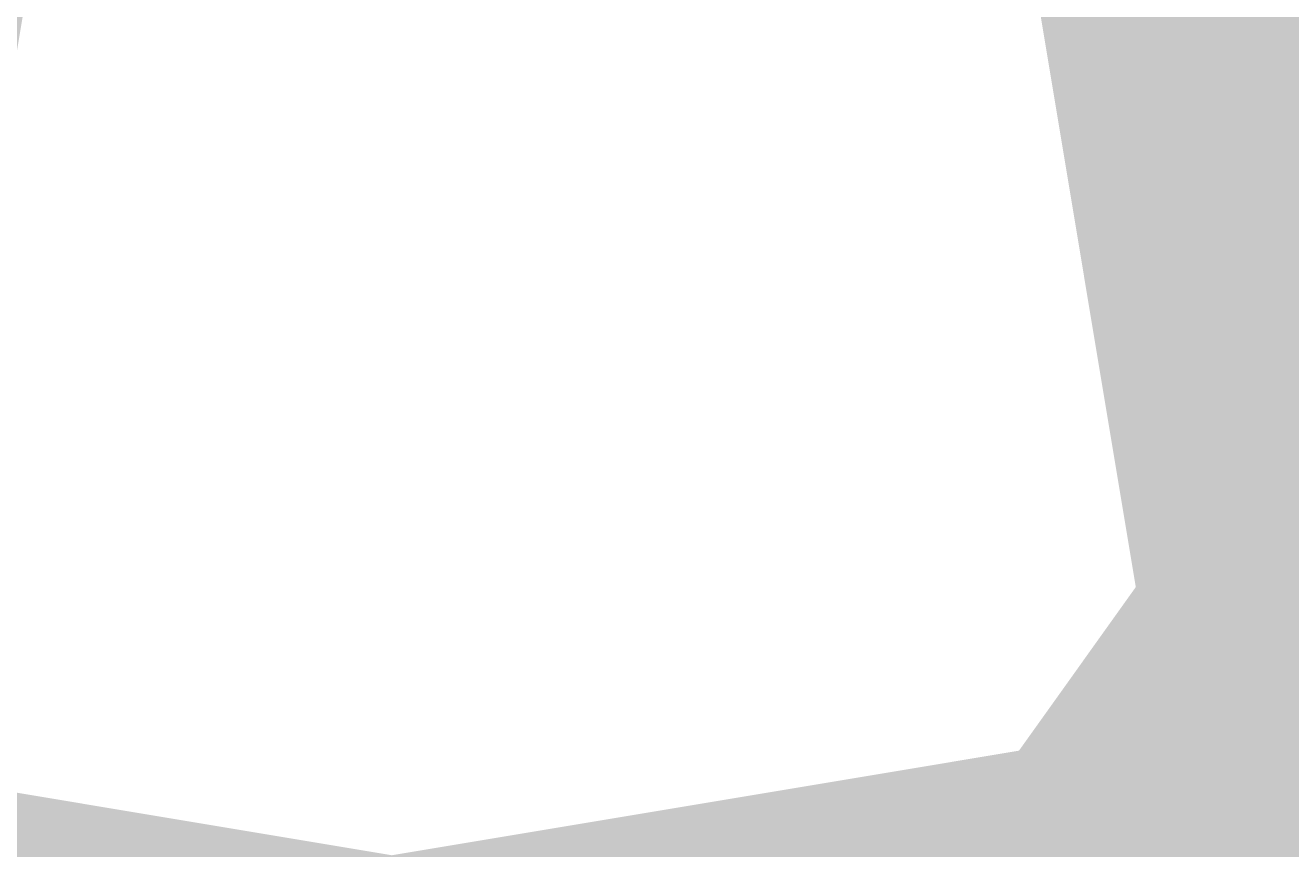
# Model space of a CAD drawing. Units: millimetres. Extents: x -22994 to 29398, y -19990 to 20176.
# Tile 122 of 135: x 99 to 296, y 213 to 341. Entities that reach past the tile are written whole.
import ezdxf

# ---------------------------------------------------------------- set-up
doc = ezdxf.new("R2010")
doc.units = ezdxf.units.MM
doc.header["$MEASUREMENT"] = 0
doc.layers.add('M-DIMS', color=2, linetype='Continuous', lineweight=18)
doc.styles.get("Standard").update_dxf_attribs({"font": 'arial.ttf'})
doc.dimstyles.get("Standard").update_dxf_attribs({"dimtxt": 0.18, "dimasz": 10000, "dimexe": 0.18, "dimexo": 0.0625, "dimgap": 0.09, "dimtad": 0, "dimtih": 1, "dimtoh": 1, "dimdec": 0, "dimzin": 0, "dimdsep": 46, "dimtxsty": 'Standard', "dimcen": 0.09, "dimadec": 0, "dimazin": 0, "dimtfac": 1, "dimtdec": 0, "dimtofl": 0, "dimtmove": 0, "dimatfit": 3, "dimfxl": 1, "dimtolj": 1, "dimtzin": 0, "dimlwd": 30, "dimarcsym": 0})

# ---------------------------------------------------------------- blocks, each defined once
blk = doc.blocks.new('*D2')
at = {"layer": 'Defpoints', "color": 0, "transparency": 16777216}
for p in [(6.68, 10.27), (290.85, 10.27), (290.85, -5.08)]:
    blk.add_point(p, dxfattribs=at)
at = {"layer": 'M-DIMS', "color": 0, "lineweight": -2, "transparency": 16777216}
for p, q in [((6.68, 10.21), (6.68, -5.26)), ((290.85, 10.21), (290.85, -5.26))]:
    blk.add_line(p, q, dxfattribs=at)
at = {"layer": 'M-DIMS', "color": 0, "lineweight": 30, "transparency": 16777216}
for p, q in [((-9993.32, -5.08), (-19993.32, -5.08)), ((10290.85, -5.08), (20290.85, -5.08))]:
    blk.add_line(p, q, dxfattribs=at)
at = {"layer": 'M-DIMS', "color": 0, "transparency": 16777216}
for points in [[(-9993.32, 1661.59), (-9993.32, -1671.75), (6.68, -5.08)], [(10290.85, 1661.59), (10290.85, -1671.75), (290.85, -5.08)]]:
    blk.add_solid(points, dxfattribs=at)
at = {"layer": 'M-DIMS', "color": 0, "transparency": 16777216, "insert": (148.76, -5.08), "char_height": 0.18, "attachment_point": 5}
blk.add_mtext('\\A1;284.2', dxfattribs=at)
blk = doc.blocks.new('*D3')
at = {"layer": 'Defpoints', "color": 0, "transparency": 16777216}
for p in [(110.26, 204.17), (110.26, 176.37), (95.83, 127.97)]:
    blk.add_point(p, dxfattribs=at)
at = {"layer": 'M-DIMS', "color": 0, "lineweight": 30, "transparency": 16777216}
for p, q in [((-9904.17, 204.17), (-19904.17, 204.17)), ((10110.26, 204.17), (20110.26, 204.17))]:
    blk.add_line(p, q, dxfattribs=at)
at = {"layer": 'M-DIMS', "color": 0, "lineweight": -2, "transparency": 16777216}
for p, q in [((95.83, 128.03), (95.83, 204.35)), ((110.26, 176.43), (110.26, 204.35))]:
    blk.add_line(p, q, dxfattribs=at)
at = {"layer": 'M-DIMS', "color": 0, "transparency": 16777216}
for points in [[(-9904.17, 1870.83), (-9904.17, -1462.5), (95.83, 204.17)], [(10110.26, 1870.83), (10110.26, -1462.5), (110.26, 204.17)]]:
    blk.add_solid(points, dxfattribs=at)
at = {"layer": 'M-DIMS', "color": 0, "transparency": 16777216, "insert": (103.05, 204.17), "char_height": 0.18, "attachment_point": 5}
blk.add_mtext('\\A1;14.432', dxfattribs=at)
blk = doc.blocks.new('*D4')
at = {"layer": 'Defpoints', "color": 0, "transparency": 16777216}
for p in [(116.26, 204.17), (110.26, 176.37), (116.26, 176.37)]:
    blk.add_point(p, dxfattribs=at)
at = {"layer": 'M-DIMS', "color": 0, "lineweight": 30, "transparency": 16777216}
for p, q in [((-9889.74, 204.17), (-19889.74, 204.17)), ((10116.26, 204.17), (20116.26, 204.17))]:
    blk.add_line(p, q, dxfattribs=at)
at = {"layer": 'M-DIMS', "color": 0, "lineweight": -2, "transparency": 16777216}
for p, q in [((110.26, 176.43), (110.26, 204.35)), ((116.26, 176.43), (116.26, 204.35))]:
    blk.add_line(p, q, dxfattribs=at)
at = {"layer": 'M-DIMS', "color": 0, "transparency": 16777216}
for points in [[(-9889.74, 1870.83), (-9889.74, -1462.5), (110.26, 204.17)], [(10116.26, 1870.83), (10116.26, -1462.5), (116.26, 204.17)]]:
    blk.add_solid(points, dxfattribs=at)
at = {"layer": 'M-DIMS', "color": 0, "transparency": 16777216, "insert": (113.26, 204.17), "char_height": 0.18, "attachment_point": 5}
blk.add_mtext('\\A1;6', dxfattribs=at)
blk = doc.blocks.new('*D5')
at = {"layer": 'Defpoints', "color": 0, "transparency": 16777216}
for p in [(181.26, 204.17), (116.26, 176.37), (181.26, 176.37)]:
    blk.add_point(p, dxfattribs=at)
at = {"layer": 'M-DIMS', "color": 0, "lineweight": 30, "transparency": 16777216}
for p, q in [((-9883.74, 204.17), (-19883.74, 204.17)), ((10181.26, 204.17), (20181.26, 204.17))]:
    blk.add_line(p, q, dxfattribs=at)
at = {"layer": 'M-DIMS', "color": 0, "lineweight": -2, "transparency": 16777216}
for p, q in [((116.26, 176.43), (116.26, 204.35)), ((181.26, 176.43), (181.26, 204.35))]:
    blk.add_line(p, q, dxfattribs=at)
at = {"layer": 'M-DIMS', "color": 0, "transparency": 16777216}
for points in [[(-9883.74, 1870.83), (-9883.74, -1462.5), (116.26, 204.17)], [(10181.26, 1870.83), (10181.26, -1462.5), (181.26, 204.17)]]:
    blk.add_solid(points, dxfattribs=at)
at = {"layer": 'M-DIMS', "color": 0, "transparency": 16777216, "insert": (148.76, 204.17), "char_height": 0.18, "attachment_point": 5}
blk.add_mtext('\\A1;65', dxfattribs=at)
blk = doc.blocks.new('*D6')
at = {"layer": 'Defpoints', "color": 0, "transparency": 16777216}
for p in [(187.26, 204.17), (181.26, 176.37), (187.26, 176.37)]:
    blk.add_point(p, dxfattribs=at)
at = {"layer": 'M-DIMS', "color": 0, "lineweight": 30, "transparency": 16777216}
for p, q in [((-9818.74, 204.17), (-19818.74, 204.17)), ((10187.26, 204.17), (20187.26, 204.17))]:
    blk.add_line(p, q, dxfattribs=at)
at = {"layer": 'M-DIMS', "color": 0, "lineweight": -2, "transparency": 16777216}
for p, q in [((181.26, 176.43), (181.26, 204.35)), ((187.26, 176.43), (187.26, 204.35))]:
    blk.add_line(p, q, dxfattribs=at)
at = {"layer": 'M-DIMS', "color": 0, "transparency": 16777216}
for points in [[(-9818.74, 1870.83), (-9818.74, -1462.5), (181.26, 204.17)], [(10187.26, 1870.83), (10187.26, -1462.5), (187.26, 204.17)]]:
    blk.add_solid(points, dxfattribs=at)
at = {"layer": 'M-DIMS', "color": 0, "transparency": 16777216, "insert": (184.26, 204.17), "char_height": 0.18, "attachment_point": 5}
blk.add_mtext('\\A1;6', dxfattribs=at)
blk = doc.blocks.new('*D7')
at = {"layer": 'Defpoints', "color": 0, "transparency": 16777216}
for p in [(201.7, 204.17), (187.26, 176.37), (201.7, 127.97)]:
    blk.add_point(p, dxfattribs=at)
at = {"layer": 'M-DIMS', "color": 0, "lineweight": 30, "transparency": 16777216}
for p, q in [((-9812.74, 204.17), (-19812.74, 204.17)), ((10201.7, 204.17), (20201.7, 204.17))]:
    blk.add_line(p, q, dxfattribs=at)
at = {"layer": 'M-DIMS', "color": 0, "lineweight": -2, "transparency": 16777216}
for p, q in [((187.26, 176.43), (187.26, 204.35)), ((201.7, 128.03), (201.7, 204.35))]:
    blk.add_line(p, q, dxfattribs=at)
at = {"layer": 'M-DIMS', "color": 0, "transparency": 16777216}
for points in [[(-9812.74, 1870.83), (-9812.74, -1462.5), (187.26, 204.17)], [(10201.7, 1870.83), (10201.7, -1462.5), (201.7, 204.17)]]:
    blk.add_solid(points, dxfattribs=at)
at = {"layer": 'M-DIMS', "color": 0, "transparency": 16777216, "insert": (194.48, 204.17), "char_height": 0.18, "attachment_point": 5}
blk.add_mtext('\\A1;14.432', dxfattribs=at)
blk = doc.blocks.new('*D8')
at = {"layer": 'Defpoints', "color": 0, "transparency": 16777216}
for p in [(227.65, 204.17), (227.65, 146.73), (201.7, 127.97)]:
    blk.add_point(p, dxfattribs=at)
at = {"layer": 'M-DIMS', "color": 0, "lineweight": 30, "transparency": 16777216}
for p, q in [((-9798.3, 204.17), (-19798.3, 204.17)), ((10227.65, 204.17), (20227.65, 204.17))]:
    blk.add_line(p, q, dxfattribs=at)
at = {"layer": 'M-DIMS', "color": 0, "lineweight": -2, "transparency": 16777216}
for p, q in [((201.7, 128.03), (201.7, 204.35)), ((227.65, 146.79), (227.65, 204.35))]:
    blk.add_line(p, q, dxfattribs=at)
at = {"layer": 'M-DIMS', "color": 0, "transparency": 16777216}
for points in [[(-9798.3, 1870.83), (-9798.3, -1462.5), (201.7, 204.17)], [(10227.65, 1870.83), (10227.65, -1462.5), (227.65, 204.17)]]:
    blk.add_solid(points, dxfattribs=at)
at = {"layer": 'M-DIMS', "color": 0, "transparency": 16777216, "insert": (214.67, 204.17), "char_height": 0.18, "attachment_point": 5}
blk.add_mtext('\\A1;25.95', dxfattribs=at)
blk = doc.blocks.new('*D9')
at = {"layer": 'Defpoints', "color": 0, "transparency": 16777216}
for p in [(187.26, 176.37), (306.2, 176.37), (290.85, 10.27)]:
    blk.add_point(p, dxfattribs=at)
at = {"layer": 'M-DIMS', "color": 0, "lineweight": 30, "transparency": 16777216}
for p, q in [((306.2, 10176.37), (306.2, 20176.37)), ((306.2, -9989.73), (306.2, -19989.73))]:
    blk.add_line(p, q, dxfattribs=at)
at = {"layer": 'M-DIMS', "color": 0, "lineweight": -2, "transparency": 16777216}
for p, q in [((187.33, 176.37), (306.38, 176.37)), ((290.91, 10.27), (306.38, 10.27))]:
    blk.add_line(p, q, dxfattribs=at)
at = {"layer": 'M-DIMS', "color": 0, "transparency": 16777216}
for points in [[(-1360.46, 10176.37), (1972.87, 10176.37), (306.2, 176.37)], [(-1360.46, -9989.73), (1972.87, -9989.73), (306.2, 10.27)]]:
    blk.add_solid(points, dxfattribs=at)
at = {"layer": 'M-DIMS', "color": 0, "transparency": 16777216, "insert": (306.2, 93.32), "char_height": 0.18, "attachment_point": 5}
blk.add_mtext('\\A1;166.1', dxfattribs=at)
blk = doc.blocks.new('*D10')
at = {"layer": 'Defpoints', "color": 0, "transparency": 16777216}
for p in [(125.65, 136.07), (133.35, 136.07), (133.35, -5.08)]:
    blk.add_point(p, dxfattribs=at)
at = {"layer": 'M-DIMS', "color": 0, "lineweight": -2, "transparency": 16777216}
for p, q in [((125.65, 136.01), (125.65, -5.26)), ((133.35, 136.01), (133.35, -5.26))]:
    blk.add_line(p, q, dxfattribs=at)
at = {"layer": 'M-DIMS', "color": 0, "lineweight": 30, "transparency": 16777216}
for p, q in [((-9874.35, -5.08), (-19874.35, -5.08)), ((10133.35, -5.08), (20133.35, -5.08))]:
    blk.add_line(p, q, dxfattribs=at)
at = {"layer": 'M-DIMS', "color": 0, "transparency": 16777216}
for points in [[(-9874.35, 1661.59), (-9874.35, -1671.75), (125.65, -5.08)], [(10133.35, 1661.59), (10133.35, -1671.75), (133.35, -5.08)]]:
    blk.add_solid(points, dxfattribs=at)
at = {"layer": 'M-DIMS', "color": 0, "transparency": 16777216, "insert": (129.5, -5.08), "char_height": 0.18, "attachment_point": 5}
blk.add_mtext('\\A1;7.696', dxfattribs=at)
blk = doc.blocks.new('*D11')
at = {"layer": 'Defpoints', "color": 0, "transparency": 16777216}
for p in [(133.35, 136.07), (135.65, 136.07), (135.65, -5.08)]:
    blk.add_point(p, dxfattribs=at)
at = {"layer": 'M-DIMS', "color": 0, "lineweight": -2, "transparency": 16777216}
for p, q in [((133.35, 136.01), (133.35, -5.26)), ((135.65, 136.01), (135.65, -5.26))]:
    blk.add_line(p, q, dxfattribs=at)
at = {"layer": 'M-DIMS', "color": 0, "lineweight": 30, "transparency": 16777216}
for p, q in [((-9866.65, -5.08), (-19866.65, -5.08)), ((10135.65, -5.08), (20135.65, -5.08))]:
    blk.add_line(p, q, dxfattribs=at)
at = {"layer": 'M-DIMS', "color": 0, "transparency": 16777216}
for points in [[(-9866.65, 1661.59), (-9866.65, -1671.75), (133.35, -5.08)], [(10135.65, 1661.59), (10135.65, -1671.75), (135.65, -5.08)]]:
    blk.add_solid(points, dxfattribs=at)
at = {"layer": 'M-DIMS', "color": 0, "transparency": 16777216, "insert": (134.5, -5.08), "char_height": 0.18, "attachment_point": 5}
blk.add_mtext('\\A1;2.304', dxfattribs=at)
blk = doc.blocks.new('*D12')
at = {"layer": 'Defpoints', "color": 0, "transparency": 16777216}
for p in [(135.65, 136.07), (145.65, 136.07), (145.65, -5.08)]:
    blk.add_point(p, dxfattribs=at)
at = {"layer": 'M-DIMS', "color": 0, "lineweight": -2, "transparency": 16777216}
for p, q in [((135.65, 136.01), (135.65, -5.26)), ((145.65, 136.01), (145.65, -5.26))]:
    blk.add_line(p, q, dxfattribs=at)
at = {"layer": 'M-DIMS', "color": 0, "lineweight": 30, "transparency": 16777216}
for p, q in [((-9864.35, -5.08), (-19864.35, -5.08)), ((10145.65, -5.08), (20145.65, -5.08))]:
    blk.add_line(p, q, dxfattribs=at)
at = {"layer": 'M-DIMS', "color": 0, "transparency": 16777216}
for points in [[(-9864.35, 1661.59), (-9864.35, -1671.75), (135.65, -5.08)], [(10145.65, 1661.59), (10145.65, -1671.75), (145.65, -5.08)]]:
    blk.add_solid(points, dxfattribs=at)
at = {"layer": 'M-DIMS', "color": 0, "transparency": 16777216, "insert": (140.65, -5.08), "char_height": 0.18, "attachment_point": 5}
blk.add_mtext('\\A1;10', dxfattribs=at)
blk = doc.blocks.new('*D13')
at = {"layer": 'Defpoints', "color": 0, "transparency": 16777216}
for p in [(145.65, 136.07), (155.65, 136.07), (155.65, -5.08)]:
    blk.add_point(p, dxfattribs=at)
at = {"layer": 'M-DIMS', "color": 0, "lineweight": -2, "transparency": 16777216}
for p, q in [((145.65, 136.01), (145.65, -5.26)), ((155.65, 136.01), (155.65, -5.26))]:
    blk.add_line(p, q, dxfattribs=at)
at = {"layer": 'M-DIMS', "color": 0, "lineweight": 30, "transparency": 16777216}
for p, q in [((-9854.35, -5.08), (-19854.35, -5.08)), ((10155.65, -5.08), (20155.65, -5.08))]:
    blk.add_line(p, q, dxfattribs=at)
at = {"layer": 'M-DIMS', "color": 0, "transparency": 16777216}
for points in [[(-9854.35, 1661.59), (-9854.35, -1671.75), (145.65, -5.08)], [(10155.65, 1661.59), (10155.65, -1671.75), (155.65, -5.08)]]:
    blk.add_solid(points, dxfattribs=at)
at = {"layer": 'M-DIMS', "color": 0, "transparency": 16777216, "insert": (150.65, -5.08), "char_height": 0.18, "attachment_point": 5}
blk.add_mtext('\\A1;10', dxfattribs=at)
blk = doc.blocks.new('*D14')
at = {"layer": 'Defpoints', "color": 0, "transparency": 16777216}
for p in [(155.65, 136.07), (165.65, 136.07), (165.65, -5.08)]:
    blk.add_point(p, dxfattribs=at)
at = {"layer": 'M-DIMS', "color": 0, "lineweight": -2, "transparency": 16777216}
for p, q in [((155.65, 136.01), (155.65, -5.26)), ((165.65, 136.01), (165.65, -5.26))]:
    blk.add_line(p, q, dxfattribs=at)
at = {"layer": 'M-DIMS', "color": 0, "lineweight": 30, "transparency": 16777216}
for p, q in [((-9844.35, -5.08), (-19844.35, -5.08)), ((10165.65, -5.08), (20165.65, -5.08))]:
    blk.add_line(p, q, dxfattribs=at)
at = {"layer": 'M-DIMS', "color": 0, "transparency": 16777216}
for points in [[(-9844.35, 1661.59), (-9844.35, -1671.75), (155.65, -5.08)], [(10165.65, 1661.59), (10165.65, -1671.75), (165.65, -5.08)]]:
    blk.add_solid(points, dxfattribs=at)
at = {"layer": 'M-DIMS', "color": 0, "transparency": 16777216, "insert": (160.65, -5.08), "char_height": 0.18, "attachment_point": 5}
blk.add_mtext('\\A1;10', dxfattribs=at)
blk = doc.blocks.new('*D15')
at = {"layer": 'Defpoints', "color": 0, "transparency": 16777216}
for p in [(173.35, 154.79), (173.35, 136.07), (306.2, 136.07)]:
    blk.add_point(p, dxfattribs=at)
at = {"layer": 'M-DIMS', "color": 0, "lineweight": 30, "transparency": 16777216}
for p, q in [((306.2, 10154.79), (306.2, 20154.79)), ((306.2, -9863.93), (306.2, -19863.93))]:
    blk.add_line(p, q, dxfattribs=at)
at = {"layer": 'M-DIMS', "color": 0, "lineweight": -2, "transparency": 16777216}
for p, q in [((173.41, 154.79), (306.38, 154.79)), ((173.41, 136.07), (306.38, 136.07))]:
    blk.add_line(p, q, dxfattribs=at)
at = {"layer": 'M-DIMS', "color": 0, "transparency": 16777216}
for points in [[(-1360.46, 10154.79), (1972.87, 10154.79), (306.2, 154.79)], [(-1360.46, -9863.93), (1972.87, -9863.93), (306.2, 136.07)]]:
    blk.add_solid(points, dxfattribs=at)
at = {"layer": 'M-DIMS', "color": 0, "transparency": 16777216, "insert": (306.2, 145.43), "char_height": 0.18, "attachment_point": 5}
blk.add_mtext('\\A1;18.717', dxfattribs=at)
blk = doc.blocks.new('*D16')
at = {"layer": 'Defpoints', "color": 0, "transparency": 16777216}
for p in [(120.17, 204.17), (110.47, 48.03), (120.17, 48.03)]:
    blk.add_point(p, dxfattribs=at)
at = {"layer": 'M-DIMS', "color": 0, "lineweight": 30, "transparency": 16777216}
for p, q in [((-9889.53, 204.17), (-19889.53, 204.17)), ((10120.17, 204.17), (20120.17, 204.17))]:
    blk.add_line(p, q, dxfattribs=at)
at = {"layer": 'M-DIMS', "color": 0, "lineweight": -2, "transparency": 16777216}
for p, q in [((110.47, 48.1), (110.47, 204.35)), ((120.17, 48.1), (120.17, 204.35))]:
    blk.add_line(p, q, dxfattribs=at)
at = {"layer": 'M-DIMS', "color": 0, "transparency": 16777216}
for points in [[(-9889.53, 1870.83), (-9889.53, -1462.5), (110.47, 204.17)], [(10120.17, 1870.83), (10120.17, -1462.5), (120.17, 204.17)]]:
    blk.add_solid(points, dxfattribs=at)
at = {"layer": 'M-DIMS', "color": 0, "transparency": 16777216, "insert": (115.32, 204.17), "char_height": 0.18, "attachment_point": 5}
blk.add_mtext('\\A1;9.704', dxfattribs=at)
blk = doc.blocks.new('*D17')
at = {"layer": 'Defpoints', "color": 0, "transparency": 16777216}
for p in [(126.17, 204.17), (120.17, 48.03), (126.17, 48.03)]:
    blk.add_point(p, dxfattribs=at)
at = {"layer": 'M-DIMS', "color": 0, "lineweight": 30, "transparency": 16777216}
for p, q in [((-9879.83, 204.17), (-19879.83, 204.17)), ((10126.17, 204.17), (20126.17, 204.17))]:
    blk.add_line(p, q, dxfattribs=at)
at = {"layer": 'M-DIMS', "color": 0, "lineweight": -2, "transparency": 16777216}
for p, q in [((120.17, 48.1), (120.17, 204.35)), ((126.17, 48.1), (126.17, 204.35))]:
    blk.add_line(p, q, dxfattribs=at)
at = {"layer": 'M-DIMS', "color": 0, "transparency": 16777216}
for points in [[(-9879.83, 1870.83), (-9879.83, -1462.5), (120.17, 204.17)], [(10126.17, 1870.83), (10126.17, -1462.5), (126.17, 204.17)]]:
    blk.add_solid(points, dxfattribs=at)
at = {"layer": 'M-DIMS', "color": 0, "transparency": 16777216, "insert": (123.17, 204.17), "char_height": 0.18, "attachment_point": 5}
blk.add_mtext('\\A1;6', dxfattribs=at)
blk = doc.blocks.new('*D18')
at = {"layer": 'Defpoints', "color": 0, "transparency": 16777216}
for p in [(132.17, 204.17), (126.17, 48.03), (132.17, 48.03)]:
    blk.add_point(p, dxfattribs=at)
at = {"layer": 'M-DIMS', "color": 0, "lineweight": 30, "transparency": 16777216}
for p, q in [((-9873.83, 204.17), (-19873.83, 204.17)), ((10132.17, 204.17), (20132.17, 204.17))]:
    blk.add_line(p, q, dxfattribs=at)
at = {"layer": 'M-DIMS', "color": 0, "lineweight": -2, "transparency": 16777216}
for p, q in [((126.17, 48.1), (126.17, 204.35)), ((132.17, 48.1), (132.17, 204.35))]:
    blk.add_line(p, q, dxfattribs=at)
at = {"layer": 'M-DIMS', "color": 0, "transparency": 16777216}
for points in [[(-9873.83, 1870.83), (-9873.83, -1462.5), (126.17, 204.17)], [(10132.17, 1870.83), (10132.17, -1462.5), (132.17, 204.17)]]:
    blk.add_solid(points, dxfattribs=at)
at = {"layer": 'M-DIMS', "color": 0, "transparency": 16777216, "insert": (129.17, 204.17), "char_height": 0.18, "attachment_point": 5}
blk.add_mtext('\\A1;6', dxfattribs=at)
blk = doc.blocks.new('*D19')
at = {"layer": 'Defpoints', "color": 0, "transparency": 16777216}
for p in [(138.17, 204.17), (132.17, 48.03), (138.17, 48.03)]:
    blk.add_point(p, dxfattribs=at)
at = {"layer": 'M-DIMS', "color": 0, "lineweight": 30, "transparency": 16777216}
for p, q in [((-9867.83, 204.17), (-19867.83, 204.17)), ((10138.17, 204.17), (20138.17, 204.17))]:
    blk.add_line(p, q, dxfattribs=at)
at = {"layer": 'M-DIMS', "color": 0, "lineweight": -2, "transparency": 16777216}
for p, q in [((132.17, 48.1), (132.17, 204.35)), ((138.17, 48.1), (138.17, 204.35))]:
    blk.add_line(p, q, dxfattribs=at)
at = {"layer": 'M-DIMS', "color": 0, "transparency": 16777216}
for points in [[(-9867.83, 1870.83), (-9867.83, -1462.5), (132.17, 204.17)], [(10138.17, 1870.83), (10138.17, -1462.5), (138.17, 204.17)]]:
    blk.add_solid(points, dxfattribs=at)
at = {"layer": 'M-DIMS', "color": 0, "transparency": 16777216, "insert": (135.17, 204.17), "char_height": 0.18, "attachment_point": 5}
blk.add_mtext('\\A1;6', dxfattribs=at)
blk = doc.blocks.new('*D20')
at = {"layer": 'Defpoints', "color": 0, "transparency": 16777216}
for p in [(144.17, 204.17), (138.17, 48.03), (144.17, 48.03)]:
    blk.add_point(p, dxfattribs=at)
at = {"layer": 'M-DIMS', "color": 0, "lineweight": 30, "transparency": 16777216}
for p, q in [((-9861.83, 204.17), (-19861.83, 204.17)), ((10144.17, 204.17), (20144.17, 204.17))]:
    blk.add_line(p, q, dxfattribs=at)
at = {"layer": 'M-DIMS', "color": 0, "lineweight": -2, "transparency": 16777216}
for p, q in [((138.17, 48.1), (138.17, 204.35)), ((144.17, 48.1), (144.17, 204.35))]:
    blk.add_line(p, q, dxfattribs=at)
at = {"layer": 'M-DIMS', "color": 0, "transparency": 16777216}
for points in [[(-9861.83, 1870.83), (-9861.83, -1462.5), (138.17, 204.17)], [(10144.17, 1870.83), (10144.17, -1462.5), (144.17, 204.17)]]:
    blk.add_solid(points, dxfattribs=at)
at = {"layer": 'M-DIMS', "color": 0, "transparency": 16777216, "insert": (141.17, 204.17), "char_height": 0.18, "attachment_point": 5}
blk.add_mtext('\\A1;6', dxfattribs=at)
blk = doc.blocks.new('*D21')
at = {"layer": 'Defpoints', "color": 0, "transparency": 16777216}
for p in [(149.12, 204.17), (144.17, 48.03), (149.12, 48.03)]:
    blk.add_point(p, dxfattribs=at)
at = {"layer": 'M-DIMS', "color": 0, "lineweight": 30, "transparency": 16777216}
for p, q in [((-9855.83, 204.17), (-19855.83, 204.17)), ((10149.12, 204.17), (20149.12, 204.17))]:
    blk.add_line(p, q, dxfattribs=at)
at = {"layer": 'M-DIMS', "color": 0, "lineweight": -2, "transparency": 16777216}
for p, q in [((144.17, 48.1), (144.17, 204.35)), ((149.12, 48.1), (149.12, 204.35))]:
    blk.add_line(p, q, dxfattribs=at)
at = {"layer": 'M-DIMS', "color": 0, "transparency": 16777216}
for points in [[(-9855.83, 1870.83), (-9855.83, -1462.5), (144.17, 204.17)], [(10149.12, 1870.83), (10149.12, -1462.5), (149.12, 204.17)]]:
    blk.add_solid(points, dxfattribs=at)
at = {"layer": 'M-DIMS', "color": 0, "transparency": 16777216, "insert": (146.64, 204.17), "char_height": 0.18, "attachment_point": 5}
blk.add_mtext('\\A1;4.945', dxfattribs=at)
blk = doc.blocks.new('*D22')
at = {"layer": 'Defpoints', "color": 0, "transparency": 16777216}
for p in [(149.12, 30.99), (155.12, 30.99), (155.12, -5.08)]:
    blk.add_point(p, dxfattribs=at)
at = {"layer": 'M-DIMS', "color": 0, "lineweight": -2, "transparency": 16777216}
for p, q in [((149.12, 30.93), (149.12, -5.26)), ((155.12, 30.93), (155.12, -5.26))]:
    blk.add_line(p, q, dxfattribs=at)
at = {"layer": 'M-DIMS', "color": 0, "lineweight": 30, "transparency": 16777216}
for p, q in [((-9850.88, -5.08), (-19850.88, -5.08)), ((10155.12, -5.08), (20155.12, -5.08))]:
    blk.add_line(p, q, dxfattribs=at)
at = {"layer": 'M-DIMS', "color": 0, "transparency": 16777216}
for points in [[(-9850.88, 1661.59), (-9850.88, -1671.75), (149.12, -5.08)], [(10155.12, 1661.59), (10155.12, -1671.75), (155.12, -5.08)]]:
    blk.add_solid(points, dxfattribs=at)
at = {"layer": 'M-DIMS', "color": 0, "transparency": 16777216, "insert": (152.12, -5.08), "char_height": 0.18, "attachment_point": 5}
blk.add_mtext('\\A1;6', dxfattribs=at)
blk = doc.blocks.new('*D23')
at = {"layer": 'Defpoints', "color": 0, "transparency": 16777216}
for p in [(155.12, 30.99), (161.12, 30.99), (161.12, -5.08)]:
    blk.add_point(p, dxfattribs=at)
at = {"layer": 'M-DIMS', "color": 0, "lineweight": -2, "transparency": 16777216}
for p, q in [((155.12, 30.93), (155.12, -5.26)), ((161.12, 30.93), (161.12, -5.26))]:
    blk.add_line(p, q, dxfattribs=at)
at = {"layer": 'M-DIMS', "color": 0, "lineweight": 30, "transparency": 16777216}
for p, q in [((-9844.88, -5.08), (-19844.88, -5.08)), ((10161.12, -5.08), (20161.12, -5.08))]:
    blk.add_line(p, q, dxfattribs=at)
at = {"layer": 'M-DIMS', "color": 0, "transparency": 16777216}
for points in [[(-9844.88, 1661.59), (-9844.88, -1671.75), (155.12, -5.08)], [(10161.12, 1661.59), (10161.12, -1671.75), (161.12, -5.08)]]:
    blk.add_solid(points, dxfattribs=at)
at = {"layer": 'M-DIMS', "color": 0, "transparency": 16777216, "insert": (158.12, -5.08), "char_height": 0.18, "attachment_point": 5}
blk.add_mtext('\\A1;6', dxfattribs=at)
blk = doc.blocks.new('*D24')
at = {"layer": 'Defpoints', "color": 0, "transparency": 16777216}
for p in [(161.12, 30.99), (166.44, 30.99), (166.44, -5.08)]:
    blk.add_point(p, dxfattribs=at)
at = {"layer": 'M-DIMS', "color": 0, "lineweight": -2, "transparency": 16777216}
for p, q in [((161.12, 30.93), (161.12, -5.26)), ((166.44, 30.93), (166.44, -5.26))]:
    blk.add_line(p, q, dxfattribs=at)
at = {"layer": 'M-DIMS', "color": 0, "lineweight": 30, "transparency": 16777216}
for p, q in [((-9838.88, -5.08), (-19838.88, -5.08)), ((10166.44, -5.08), (20166.44, -5.08))]:
    blk.add_line(p, q, dxfattribs=at)
at = {"layer": 'M-DIMS', "color": 0, "transparency": 16777216}
for points in [[(-9838.88, 1661.59), (-9838.88, -1671.75), (161.12, -5.08)], [(10166.44, 1661.59), (10166.44, -1671.75), (166.44, -5.08)]]:
    blk.add_solid(points, dxfattribs=at)
at = {"layer": 'M-DIMS', "color": 0, "transparency": 16777216, "insert": (163.78, -5.08), "char_height": 0.18, "attachment_point": 5}
blk.add_mtext('\\A1;5.323', dxfattribs=at)
blk = doc.blocks.new('*D25')
at = {"layer": 'Defpoints', "color": 0, "transparency": 16777216}
for p in [(166.44, 30.99), (172.44, 30.99), (172.44, -5.08)]:
    blk.add_point(p, dxfattribs=at)
at = {"layer": 'M-DIMS', "color": 0, "lineweight": -2, "transparency": 16777216}
for p, q in [((166.44, 30.93), (166.44, -5.26)), ((172.44, 30.93), (172.44, -5.26))]:
    blk.add_line(p, q, dxfattribs=at)
at = {"layer": 'M-DIMS', "color": 0, "lineweight": 30, "transparency": 16777216}
for p, q in [((-9833.56, -5.08), (-19833.56, -5.08)), ((10172.44, -5.08), (20172.44, -5.08))]:
    blk.add_line(p, q, dxfattribs=at)
at = {"layer": 'M-DIMS', "color": 0, "transparency": 16777216}
for points in [[(-9833.56, 1661.59), (-9833.56, -1671.75), (166.44, -5.08)], [(10172.44, 1661.59), (10172.44, -1671.75), (172.44, -5.08)]]:
    blk.add_solid(points, dxfattribs=at)
at = {"layer": 'M-DIMS', "color": 0, "transparency": 16777216, "insert": (169.44, -5.08), "char_height": 0.18, "attachment_point": 5}
blk.add_mtext('\\A1;6', dxfattribs=at)
blk = doc.blocks.new('*D26')
at = {"layer": 'Defpoints', "color": 0, "transparency": 16777216}
for p in [(172.44, 30.99), (178.44, 30.99), (178.44, -5.08)]:
    blk.add_point(p, dxfattribs=at)
at = {"layer": 'M-DIMS', "color": 0, "lineweight": -2, "transparency": 16777216}
for p, q in [((172.44, 30.93), (172.44, -5.26)), ((178.44, 30.93), (178.44, -5.26))]:
    blk.add_line(p, q, dxfattribs=at)
at = {"layer": 'M-DIMS', "color": 0, "lineweight": 30, "transparency": 16777216}
for p, q in [((-9827.56, -5.08), (-19827.56, -5.08)), ((10178.44, -5.08), (20178.44, -5.08))]:
    blk.add_line(p, q, dxfattribs=at)
at = {"layer": 'M-DIMS', "color": 0, "transparency": 16777216}
for points in [[(-9827.56, 1661.59), (-9827.56, -1671.75), (172.44, -5.08)], [(10178.44, 1661.59), (10178.44, -1671.75), (178.44, -5.08)]]:
    blk.add_solid(points, dxfattribs=at)
at = {"layer": 'M-DIMS', "color": 0, "transparency": 16777216, "insert": (175.44, -5.08), "char_height": 0.18, "attachment_point": 5}
blk.add_mtext('\\A1;6', dxfattribs=at)
blk = doc.blocks.new('*D27')
at = {"layer": 'Defpoints', "color": 0, "transparency": 16777216}
for p in [(178.44, 30.99), (188.12, 30.99), (188.12, -5.08)]:
    blk.add_point(p, dxfattribs=at)
at = {"layer": 'M-DIMS', "color": 0, "lineweight": -2, "transparency": 16777216}
for p, q in [((178.44, 30.93), (178.44, -5.26)), ((188.12, 30.93), (188.12, -5.26))]:
    blk.add_line(p, q, dxfattribs=at)
at = {"layer": 'M-DIMS', "color": 0, "lineweight": 30, "transparency": 16777216}
for p, q in [((-9821.56, -5.08), (-19821.56, -5.08)), ((10188.12, -5.08), (20188.12, -5.08))]:
    blk.add_line(p, q, dxfattribs=at)
at = {"layer": 'M-DIMS', "color": 0, "transparency": 16777216}
for points in [[(-9821.56, 1661.59), (-9821.56, -1671.75), (178.44, -5.08)], [(10188.12, 1661.59), (10188.12, -1671.75), (188.12, -5.08)]]:
    blk.add_solid(points, dxfattribs=at)
at = {"layer": 'M-DIMS', "color": 0, "transparency": 16777216, "insert": (183.28, -5.08), "char_height": 0.18, "attachment_point": 5}
blk.add_mtext('\\A1;9.679', dxfattribs=at)
blk = doc.blocks.new('*D28')
at = {"layer": 'Defpoints', "color": 0, "transparency": 16777216}
for p in [(188.12, 48.03), (306.2, 48.03), (188.12, 30.99)]:
    blk.add_point(p, dxfattribs=at)
at = {"layer": 'M-DIMS', "color": 0, "lineweight": 30, "transparency": 16777216}
for p, q in [((306.2, 10048.03), (306.2, 20048.03)), ((306.2, -9969.01), (306.2, -19969.01))]:
    blk.add_line(p, q, dxfattribs=at)
at = {"layer": 'M-DIMS', "color": 0, "lineweight": -2, "transparency": 16777216}
for p, q in [((188.18, 48.03), (306.38, 48.03)), ((188.18, 30.99), (306.38, 30.99))]:
    blk.add_line(p, q, dxfattribs=at)
at = {"layer": 'M-DIMS', "color": 0, "transparency": 16777216}
for points in [[(-1360.46, 10048.03), (1972.87, 10048.03), (306.2, 48.03)], [(-1360.46, -9969.01), (1972.87, -9969.01), (306.2, 30.99)]]:
    blk.add_solid(points, dxfattribs=at)
at = {"layer": 'M-DIMS', "color": 0, "transparency": 16777216, "insert": (306.2, 39.51), "char_height": 0.18, "attachment_point": 5}
blk.add_mtext('\\A1;17.045', dxfattribs=at)
blk = doc.blocks.new('*D29')
at = {"layer": 'Defpoints', "color": 0, "transparency": 16777216}
for p in [(36.8, 80.04), (64.03, 80.04)]:
    blk.add_point(p, dxfattribs=at)
at = {"layer": 'M-DIMS', "color": 0, "lineweight": -2, "transparency": 16777216}
for p, q in [((50.33, 80.04), (50.51, 80.04)), ((50.42, 79.96), (50.42, 80.14))]:
    blk.add_line(p, q, dxfattribs=at)
at = {"layer": 'M-DIMS', "color": 0, "lineweight": 30, "transparency": 16777216}
blk.add_line((20064.03, 80.03), (10064.03, 80.04), dxfattribs=at)
at = {"layer": 'M-DIMS', "color": 0, "transparency": 16777216}
blk.add_solid([(10064.03, 1746.7), (10064.03, -1586.63), (64.03, 80.04)], dxfattribs=at)
at = {"layer": 'M-DIMS', "color": 0, "transparency": 16777216, "insert": (20064.52, 80.03), "char_height": 0.18, "attachment_point": 5}
blk.add_mtext('\\A1;∅27.23', dxfattribs=at)
blk = doc.blocks.new('*D30')
at = {"layer": 'Defpoints', "color": 0, "transparency": 16777216}
for p in [(216.31, 146.73), (238.98, 146.73)]:
    blk.add_point(p, dxfattribs=at)
at = {"layer": 'M-DIMS', "color": 0, "lineweight": -2, "transparency": 16777216}
for p, q in [((227.56, 146.73), (227.74, 146.73)), ((227.65, 146.64), (227.65, 146.82))]:
    blk.add_line(p, q, dxfattribs=at)
at = {"layer": 'M-DIMS', "color": 0, "lineweight": 30, "transparency": 16777216}
blk.add_line((20238.98, 147.5), (10238.98, 147.11), dxfattribs=at)
at = {"layer": 'M-DIMS', "color": 0, "transparency": 16777216}
blk.add_solid([(10238.92, 1813.78), (10239.05, -1519.55), (238.98, 146.73)], dxfattribs=at)
at = {"layer": 'M-DIMS', "color": 0, "transparency": 16777216, "insert": (20239.54, 147.5), "char_height": 0.18, "attachment_point": 5}
blk.add_mtext('\\A1;∅22.667', dxfattribs=at)
blk = doc.blocks.new('*D31')
at = {"layer": 'Defpoints', "color": 0, "transparency": 16777216}
for p in [(223.16, 146.73), (232.13, 146.73)]:
    blk.add_point(p, dxfattribs=at)
at = {"layer": 'M-DIMS', "color": 0, "lineweight": 30, "transparency": 16777216}
blk.add_line((20232.13, 148.67), (10232.13, 147.7), dxfattribs=at)
at = {"layer": 'M-DIMS', "color": 0, "lineweight": -2, "transparency": 16777216}
for p, q in [((227.56, 146.73), (227.74, 146.73)), ((227.65, 146.64), (227.65, 146.82))]:
    blk.add_line(p, q, dxfattribs=at)
at = {"layer": 'M-DIMS', "color": 0, "transparency": 16777216}
blk.add_solid([(10231.97, 1814.36), (10232.29, -1518.97), (232.13, 146.73)], dxfattribs=at)
at = {"layer": 'M-DIMS', "color": 0, "transparency": 16777216, "insert": (20232.62, 148.67), "char_height": 0.18, "attachment_point": 5}
blk.add_mtext('\\A1;∅8.969', dxfattribs=at)
blk = doc.blocks.new('*D34')
at = {"layer": 'Defpoints', "color": 0, "transparency": 16777216}
for p in [(178.58, 122.9), (176.81, 121.13)]:
    blk.add_point(p, dxfattribs=at)
at = {"layer": 'M-DIMS', "color": 0, "lineweight": 30, "transparency": 16777216}
for p, q in [((14322.44, 14263.31), (7250.51, 7193.1)), ((24322.44, 14263.31), (14322.44, 14263.31))]:
    blk.add_line(p, q, dxfattribs=at)
at = {"layer": 'M-DIMS', "color": 0, "lineweight": -2, "transparency": 16777216}
for p, q in [((176.72, 121.13), (176.9, 121.13)), ((176.81, 121.04), (176.81, 121.22))]:
    blk.add_line(p, q, dxfattribs=at)
at = {"layer": 'M-DIMS', "color": 0, "transparency": 16777216}
blk.add_solid([(6072.14, 8371.76), (8428.88, 6014.45), (178.58, 122.9)], dxfattribs=at)
at = {"layer": 'M-DIMS', "color": 0, "transparency": 16777216, "insert": (24322.97, 14263.31), "char_height": 0.18, "attachment_point": 5}
blk.add_mtext('\\A1;6X R2.5', dxfattribs=at)
blk = doc.blocks.new('*D36')
at = {"layer": 'Defpoints', "color": 0, "transparency": 16777216}
for p in [(46.39, 31.3), (46.39, 26.59)]:
    blk.add_point(p, dxfattribs=at)
at = {"layer": 'M-DIMS', "color": 0, "lineweight": 30, "transparency": 16777216}
for p, q in [((57.15, 20031.3), (51.77, 10031.3)), ((10057.15, 20031.3), (57.15, 20031.3))]:
    blk.add_line(p, q, dxfattribs=at)
at = {"layer": 'M-DIMS', "color": 0, "lineweight": -2, "transparency": 16777216}
for p, q in [((46.3, 28.95), (46.48, 28.95)), ((46.39, 28.86), (46.39, 29.04))]:
    blk.add_line(p, q, dxfattribs=at)
at = {"layer": 'M-DIMS', "color": 0, "transparency": 16777216}
blk.add_solid([(-1614.9, 10032.2), (1718.44, 10030.41), (46.39, 31.3)], dxfattribs=at)
at = {"layer": 'M-DIMS', "color": 0, "transparency": 16777216, "insert": (10057.55, 20031.3), "char_height": 0.18, "attachment_point": 5}
blk.add_mtext('\\A1;∅4.71', dxfattribs=at)
blk = doc.blocks.new('*D37')
at = {"layer": 'Defpoints', "color": 0, "transparency": 16777216}
for p in [(54.83, 118.61), (59.49, 118.61)]:
    blk.add_point(p, dxfattribs=at)
at = {"layer": 'M-DIMS', "color": 0, "lineweight": -2, "transparency": 16777216}
for p, q in [((57.07, 118.61), (57.25, 118.61)), ((57.16, 118.52), (57.16, 118.7))]:
    blk.add_line(p, q, dxfattribs=at)
at = {"layer": 'M-DIMS', "color": 0, "lineweight": 30, "transparency": 16777216}
blk.add_line((20059.49, 116.25), (10059.49, 117.43), dxfattribs=at)
at = {"layer": 'M-DIMS', "color": 0, "transparency": 16777216}
blk.add_solid([(10059.69, 1784.1), (10059.3, -1549.23), (59.49, 118.61)], dxfattribs=at)
at = {"layer": 'M-DIMS', "color": 0, "transparency": 16777216, "insert": (20059.99, 116.25), "char_height": 0.18, "attachment_point": 5}
blk.add_mtext('\\A1;∅4.659', dxfattribs=at)

msp = doc.modelspace()

# ---------------------------------------------------------------- dimensions: what is measured, and where the dimension line sits
at = {"layer": 'M-DIMS'}
for base, p1, p2, override, picture, middle in [((306.202, 176.3662), (290.852, 10.2713), (187.2647, 176.3662), {"dimdec": 1, "dimlfac": 1, "dimrnd": 0, "dimzin": 0, "dimdsep": 46, "dimlunit": 2}, '*D9', (306.202, 93.3187)), ((306.202, 136.0713), (173.3459, 154.788), (173.3459, 136.0713), {"dimdec": 3, "dimlfac": 1, "dimrnd": 0, "dimzin": 0, "dimdsep": 46, "dimlunit": 2}, '*D15', (306.202, 145.4297)), ((306.202, 48.0349), (188.1175, 30.9895), (188.1175, 48.0349), {"dimdec": 3, "dimlfac": 1, "dimrnd": 0, "dimzin": 0, "dimdsep": 46, "dimlunit": 2}, '*D28', (306.202, 39.5122))]:
    dim = msp.add_linear_dim(base=base, p1=p1, p2=p2, angle=90, dimstyle='Standard', override=override, dxfattribs=at)
    dim.commit()
    dim.dimension.update_dxf_attribs({"geometry": picture, "text_midpoint": middle})
for p1, p2, override, picture, middle in [((46.3875, 26.5934), (46.39, 31.3035), {"dimdec": 2, "dimlfac": 1, "dimrnd": 0, "dimzin": 0, "dimdsep": 46, "dimlunit": 2}, '*D36', (10057.5542, 20031.3006)), ((216.3148, 146.7291), (238.9821, 146.73), {"dimdec": 3, "dimlfac": 1, "dimrnd": 0, "dimzin": 0, "dimdsep": 46, "dimlunit": 2}, '*D30', (20238.9821, 147.4959)), ((223.1641, 146.7291), (232.1328, 146.73), {"dimdec": 3, "dimlfac": 1, "dimrnd": 0, "dimzin": 0, "dimdsep": 46, "dimlunit": 2}, '*D31', (20232.1327, 148.6656))]:
    dim = msp.add_diameter_dim_2p(p1=p1, p2=p2, dimstyle='Standard', override=override, dxfattribs=at)
    dim.commit()
    dim.dimension.update_dxf_attribs({"geometry": picture, "text_midpoint": middle, "dimtype": 163})
dim = msp.add_radius_dim(center=(176.8123, 121.1277), mpoint=(178.5802, 122.8952), text='6X <>', dimstyle='Standard', override={"dimdec": 1, "dimlfac": 1, "dimrnd": 0, "dimzin": 0, "dimdsep": 46, "dimlunit": 2}, dxfattribs=at)
dim.commit()
dim.dimension.update_dxf_attribs({"geometry": '*D34', "text_midpoint": (24322.9703, 14263.3108)})
for base, p1, p2, override, picture, middle in [((110.2647, 204.1654), (95.8327, 127.967), (110.2647, 176.3662), {"dimdec": 3, "dimlfac": 1, "dimrnd": 0, "dimzin": 0, "dimdsep": 46, "dimlunit": 2}, '*D3', (103.0487, 204.1654)), ((116.2647, 204.1654), (110.2647, 176.3662), (116.2647, 176.3662), {"dimdec": 0, "dimlfac": 1, "dimrnd": 0, "dimzin": 0, "dimdsep": 46, "dimlunit": 2}, '*D4', (113.2647, 204.1654)), ((120.1702, 204.1654), (110.4658, 48.0349), (120.1702, 48.0349), {"dimdec": 3, "dimlfac": 1, "dimrnd": 0, "dimzin": 0, "dimdsep": 46, "dimlunit": 2}, '*D16', (115.318, 204.1654)), ((181.2647, 204.1654), (116.2647, 176.3662), (181.2647, 176.3662), {"dimdec": 0, "dimlfac": 1, "dimrnd": 0, "dimzin": 0, "dimdsep": 46, "dimlunit": 2}, '*D5', (148.7647, 204.1654)), ((126.1702, 204.1654), (120.1702, 48.0349), (126.1702, 48.0349), {"dimdec": 0, "dimlfac": 1, "dimrnd": 0, "dimzin": 0, "dimdsep": 46, "dimlunit": 2}, '*D17', (123.1702, 204.1654)), ((132.1702, 204.1654), (126.1702, 48.0349), (132.1702, 48.0349), {"dimdec": 0, "dimlfac": 1, "dimrnd": 0, "dimzin": 0, "dimdsep": 46, "dimlunit": 2}, '*D18', (129.1702, 204.1654)), ((138.1702, 204.1654), (132.1702, 48.0349), (138.1702, 48.0349), {"dimdec": 0, "dimlfac": 1, "dimrnd": 0, "dimzin": 0, "dimdsep": 46, "dimlunit": 2}, '*D19', (135.1702, 204.1654)), ((144.1702, 204.1654), (138.1702, 48.0349), (144.1702, 48.0349), {"dimdec": 0, "dimlfac": 1, "dimrnd": 0, "dimzin": 0, "dimdsep": 46, "dimlunit": 2}, '*D20', (141.1702, 204.1654)), ((149.11567, 204.16539), (144.17023, 48.03494), (149.11567, 48.03494), {"dimdec": 3, "dimlfac": 1, "dimrnd": 0, "dimzin": 0, "dimdsep": 46, "dimlunit": 2}, '*D21', (146.64295, 204.16539)), ((187.2647, 204.1654), (181.2647, 176.3662), (187.2647, 176.3662), {"dimdec": 0, "dimlfac": 1, "dimrnd": 0, "dimzin": 0, "dimdsep": 46, "dimlunit": 2}, '*D6', (184.2647, 204.1654)), ((201.6967, 204.1654), (187.2647, 176.3662), (201.6967, 127.967), {"dimdec": 3, "dimlfac": 1, "dimrnd": 0, "dimzin": 0, "dimdsep": 46, "dimlunit": 2}, '*D7', (194.4807, 204.1654)), ((227.6485, 204.1654), (201.6967, 127.967), (227.6485, 146.7296), {"dimdec": 2, "dimlfac": 1, "dimrnd": 0, "dimzin": 0, "dimdsep": 46, "dimlunit": 2}, '*D8', (214.6726, 204.1654)), ((290.852, -5.0787), (6.6773, 10.2713), (290.852, 10.2713), {"dimdec": 1, "dimlfac": 1, "dimrnd": 0, "dimzin": 0, "dimdsep": 46, "dimlunit": 2}, '*D2', (148.7647, -5.0787)), ((133.3459, -5.0787), (125.6498, 136.0713), (133.3459, 136.0713), {"dimdec": 3, "dimlfac": 1, "dimrnd": 0, "dimzin": 0, "dimdsep": 46, "dimlunit": 2}, '*D10', (129.4978, -5.0787)), ((135.6498, -5.0787), (133.3459, 136.0713), (135.6498, 136.0713), {"dimdec": 3, "dimlfac": 1, "dimrnd": 0, "dimzin": 0, "dimdsep": 46, "dimlunit": 2}, '*D11', (134.4978, -5.0787)), ((145.6498, -5.0787), (135.6498, 136.0713), (145.6498, 136.0713), {"dimdec": 0, "dimlfac": 1, "dimrnd": 0, "dimzin": 0, "dimdsep": 46, "dimlunit": 2}, '*D12', (140.6498, -5.0787)), ((155.6498, -5.0787), (145.6498, 136.0713), (155.6498, 136.0713), {"dimdec": 0, "dimlfac": 1, "dimrnd": 0, "dimzin": 0, "dimdsep": 46, "dimlunit": 2}, '*D13', (150.6498, -5.0787)), ((155.1157, -5.0787), (149.1157, 30.9895), (155.1157, 30.9895), {"dimdec": 0, "dimlfac": 1, "dimrnd": 0, "dimzin": 0, "dimdsep": 46, "dimlunit": 2}, '*D22', (152.1157, -5.0787)), ((161.1157, -5.0787), (155.1157, 30.9895), (161.1157, 30.9895), {"dimdec": 0, "dimlfac": 1, "dimrnd": 0, "dimzin": 0, "dimdsep": 46, "dimlunit": 2}, '*D23', (158.1157, -5.0787)), ((165.6498, -5.0787), (155.6498, 136.0713), (165.6498, 136.0713), {"dimdec": 0, "dimlfac": 1, "dimrnd": 0, "dimzin": 0, "dimdsep": 46, "dimlunit": 2}, '*D14', (160.6498, -5.0787)), ((166.4387, -5.0787), (161.1157, 30.9895), (166.4387, 30.9895), {"dimdec": 3, "dimlfac": 1, "dimrnd": 0, "dimzin": 0, "dimdsep": 46, "dimlunit": 2}, '*D24', (163.7772, -5.0787)), ((172.4387, -5.0787), (166.4387, 30.9895), (172.4387, 30.9895), {"dimdec": 0, "dimlfac": 1, "dimrnd": 0, "dimzin": 0, "dimdsep": 46, "dimlunit": 2}, '*D25', (169.4387, -5.0787)), ((178.4387, -5.0787), (172.4387, 30.9895), (178.4387, 30.9895), {"dimdec": 0, "dimlfac": 1, "dimrnd": 0, "dimzin": 0, "dimdsep": 46, "dimlunit": 2}, '*D26', (175.4387, -5.0787)), ((188.1175, -5.0787), (178.4387, 30.9895), (188.1175, 30.9895), {"dimdec": 3, "dimlfac": 1, "dimrnd": 0, "dimzin": 0, "dimdsep": 46, "dimlunit": 2}, '*D27', (183.2781, -5.0787))]:
    dim = msp.add_linear_dim(base=base, p1=p1, p2=p2, dimstyle='Standard', override=override, dxfattribs=at)
    dim.commit()
    dim.dimension.update_dxf_attribs({"geometry": picture, "text_midpoint": middle})
for p1, p2, override, picture, middle in [((54.8343, 118.6145), (59.4936, 118.614), {"dimdec": 3, "dimlfac": 1, "dimrnd": 0, "dimzin": 0, "dimdsep": 46, "dimlunit": 2}, '*D37', (20059.4934, 116.2531)), ((36.8006, 80.045), (64.0296, 80.045), {"dimdec": 2, "dimlfac": 1, "dimrnd": 0, "dimzin": 0, "dimdsep": 46, "dimlunit": 2}, '*D29', (20064.0296, 80.0303))]:
    dim = msp.add_diameter_dim_2p(p1=p1, p2=p2, dimstyle='Standard', override=override, dxfattribs=at)
    dim.commit()
    dim.dimension.update_dxf_attribs({"geometry": picture, "text_midpoint": middle})

doc.saveas('drawing.dxf')
